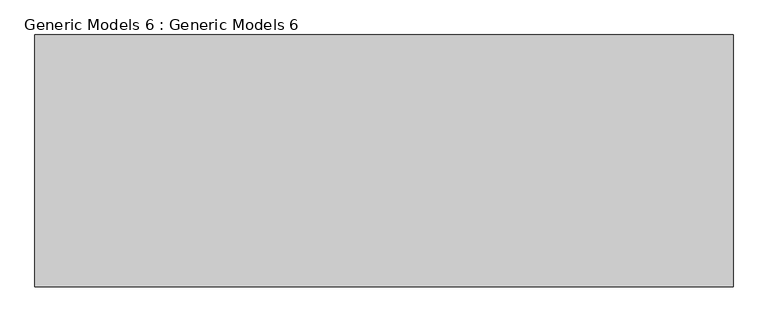
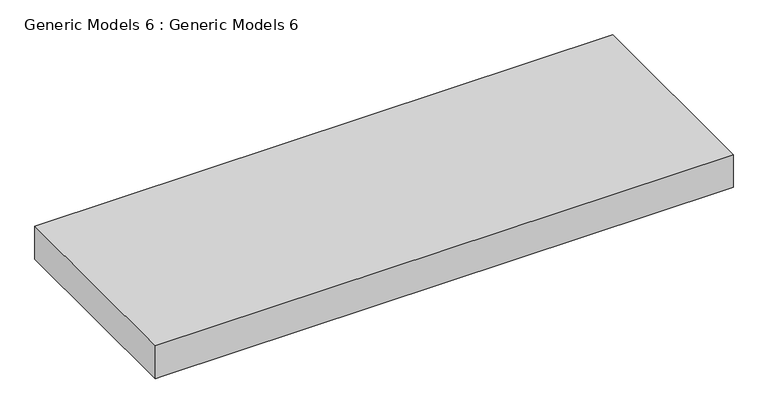
"""IFC4 building model written with IfcOpenShell, lengths in millimetres: proxy geometry, Generic Models 6 : Generic Models 6."""

from ifc_helpers import new_model, si_unit, frame, origin, place, context, project, spatial, polyline, outline, extrude, source, transform, mapped, element, save


def generic_models_6_generic_models_6_bff87668(model_context):
    return source(origin(), model_context, "Body", "SweptSolid", [
        extrude(outline(polyline([(5238.75, -5275.4019453), (5340.35, -5275.4019453), (5340.35, -6964.5019453), (5238.75, -6964.5019453), (5238.75, -6939.1019453), (5238.75, -5300.8019453), (5238.75, -5275.4019453)])), frame((0.0, 3362.4444012, 0.0), z_axis=(0.0, 1.0, 0.0), x_axis=(0.0, 0.0, 1.0)), (0.0, 0.0, 1.0), 609.6),
    ])


if __name__ == "__main__":
    model = new_model("IFC4")
    model_context = context("Model", 3, world=origin())
    ifc_project = project(units=[si_unit("LENGTHUNIT", "METRE", prefix="MILLI")], contexts=[model_context])
    site = spatial("IfcSite", under=ifc_project)
    building = spatial("IfcBuilding", under=site)
    placement = place(None, origin())
    generic_models_6_generic_models_6_shape = generic_models_6_generic_models_6_bff87668(model_context)
    element("IfcBuildingElementProxy", 1, Name="Generic Models 6 : Generic Models 6", ObjectType="Generic Models 6 : Generic Models 6", at=placement, inside=building, context=model_context, shape_type="MappedRepresentation", body=[
        mapped(generic_models_6_generic_models_6_shape, transform((0.0, 0.0, 0.0), x_axis=(1.0, 0.0, 0.0), y_axis=(0.0, 1.0, 0.0), z_axis=(0.0, 0.0, 1.0))),
    ])
    save(model, "model.ifc")
